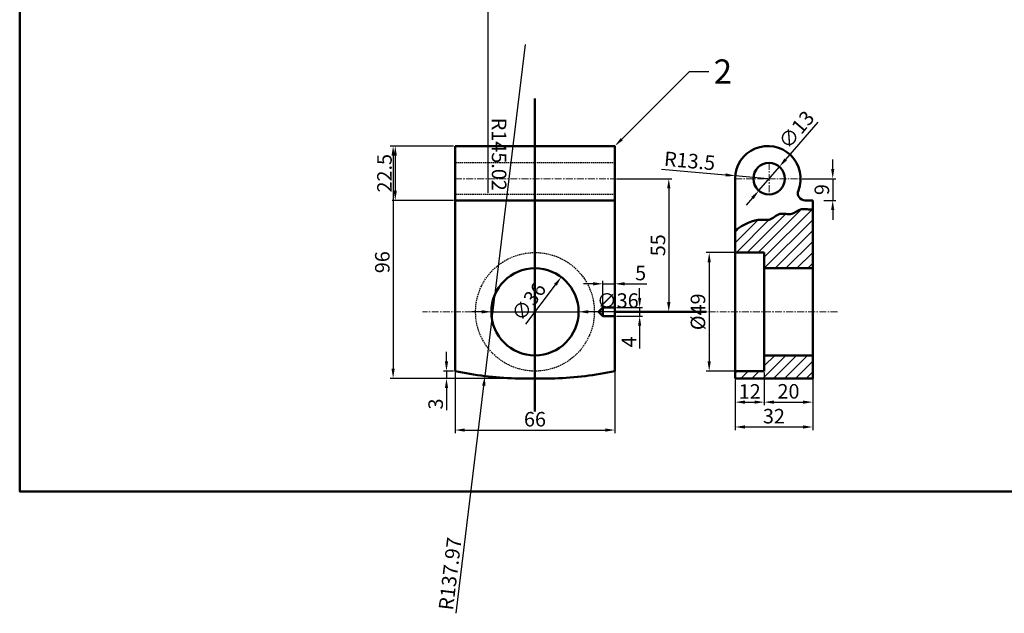
# Model space of a CAD drawing. Units: millimetres. Extents: x 197 to 841, y -182 to 351.
# Tile 1 of 3: x 197 to 603, y -182 to 63. Entities that reach past the tile are written whole.
import ezdxf
from ezdxf import colors
from ezdxf.entities.mleader import LeaderData, LeaderLine
from ezdxf.math import Vec2, Vec3

# ---------------------------------------------------------------- set-up
doc = ezdxf.new("R2010")
doc.units = ezdxf.units.MM
doc.header["$LTSCALE"] = 0.3
doc.linetypes.add('CENTER', pattern=[50.8, 31.75, -6.35, 6.35, -6.35])
doc.linetypes.add('HIDDEN', pattern=[9.525, 6.35, -3.175])
for name, color, linetype, lineweight in [('M-CNTR', 1, 'CENTER', 18), ('M-DIMS', 2, 'Continuous', 25), ('M-HATC', 8, 'Continuous', 18), ('M-HIDN', 6, 'HIDDEN', 25), ('M-OUTL', 7, 'Continuous', 50), ('M-TTLB', 7, 'Continuous', 50)]:
    doc.layers.add(name, color=color, linetype=linetype, lineweight=lineweight)
doc.styles.get("Standard").update_dxf_attribs({"font": 'arial.ttf'})
doc.dimstyles.new('ISO-25', dxfattribs={"dimtxt": 6, "dimasz": 4, "dimexe": 1.25, "dimexo": 0.625, "dimtad": 1, "dimdec": 0, "dimtxsty": 'Standard', "dimcen": 2.5, "dimadec": 0, "dimazin": 0, "dimtfac": 1, "dimtdec": 0, "dimtmove": 0, "dimatfit": 3, "dimfxl": 1, "dimarcsym": 0})

# ---------------------------------------------------------------- blocks, each defined once
blk = doc.blocks.new('*D24')
at = {"layer": 'Defpoints', "color": 0, "ltscale": 0.3, "transparency": 16777216}
for p in [(376.21, 11.02), (350.66, -84.98), (409.21, -84.98)]:
    blk.add_point(p, dxfattribs=at)
at = {"layer": 'M-DIMS', "color": 0, "lineweight": -2, "ltscale": 0.3, "transparency": 16777216}
for p, q in [((375.58, 11.02), (349.41, 11.02)), ((350.66, 7.02), (350.66, -80.98)), ((408.58, -84.98), (349.41, -84.98))]:
    blk.add_line(p, q, dxfattribs=at)
at = {"layer": 'M-DIMS', "color": 0, "ltscale": 0.3, "transparency": 16777216}
for points in [[(349.99, 7.02), (351.32, 7.02), (350.66, 11.02)], [(349.99, -80.98), (351.32, -80.98), (350.66, -84.98)]]:
    blk.add_solid(points, dxfattribs=at)
at = {"layer": 'M-DIMS', "color": 0, "ltscale": 0.3, "transparency": 16777216, "insert": (346.97, -36.98), "char_height": 6, "attachment_point": 5, "rotation": 90}
blk.add_mtext('96', dxfattribs=at)
blk = doc.blocks.new('*D25')
at = {"layer": 'Defpoints', "color": 0, "ltscale": 0.3, "transparency": 16777216}
for p in [(376.21, -72.47), (442.21, -72.47), (442.21, -106.33)]:
    blk.add_point(p, dxfattribs=at)
at = {"layer": 'M-DIMS', "color": 0, "lineweight": -2, "ltscale": 0.3, "transparency": 16777216}
for p, q in [((376.21, -73.1), (376.21, -107.58)), ((442.21, -73.1), (442.21, -107.58)), ((380.21, -106.33), (438.21, -106.33))]:
    blk.add_line(p, q, dxfattribs=at)
at = {"layer": 'M-DIMS', "color": 0, "ltscale": 0.3, "transparency": 16777216}
for points in [[(380.21, -105.66), (380.21, -107), (376.21, -106.33)], [(438.21, -105.66), (438.21, -107), (442.21, -106.33)]]:
    blk.add_solid(points, dxfattribs=at)
at = {"layer": 'M-DIMS', "color": 0, "ltscale": 0.3, "transparency": 16777216, "insert": (409.21, -102.64), "char_height": 6, "attachment_point": 5}
blk.add_mtext('66', dxfattribs=at)
blk = doc.blocks.new('*D26')
at = {"layer": 'Defpoints', "color": 0, "ltscale": 0.3, "transparency": 16777216}
for p in [(442.21, -55.73), (442.21, -59.23), (452.41, -59.23)]:
    blk.add_point(p, dxfattribs=at)
at = {"layer": 'M-DIMS', "color": 0, "lineweight": -2, "ltscale": 0.3, "transparency": 16777216}
for p, q in [((452.41, -51.73), (452.41, -47.73)), ((442.83, -55.73), (453.66, -55.73)), ((452.41, -55.73), (452.41, -59.23)), ((442.83, -59.23), (453.66, -59.23)), ((452.41, -63.23), (452.41, -72.63))]:
    blk.add_line(p, q, dxfattribs=at)
at = {"layer": 'M-DIMS', "color": 0, "ltscale": 0.3, "transparency": 16777216}
for points in [[(451.75, -51.73), (453.08, -51.73), (452.41, -55.73)], [(451.75, -63.23), (453.08, -63.23), (452.41, -59.23)]]:
    blk.add_solid(points, dxfattribs=at)
at = {"layer": 'M-DIMS', "color": 0, "ltscale": 0.3, "transparency": 16777216, "insert": (448.79, -69.93), "char_height": 6, "attachment_point": 5, "rotation": 90}
blk.add_mtext('4', dxfattribs=at)
blk = doc.blocks.new('*D27')
at = {"layer": 'Defpoints', "color": 0, "ltscale": 0.3, "transparency": 16777216}
for p in [(442.21, -45.91), (437.21, -57.48), (442.21, -57.48)]:
    blk.add_point(p, dxfattribs=at)
at = {"layer": 'M-DIMS', "color": 0, "lineweight": -2, "ltscale": 0.3, "transparency": 16777216}
for p, q in [((437.21, -56.85), (437.21, -44.66)), ((442.21, -56.85), (442.21, -44.66)), ((433.21, -45.91), (429.21, -45.91)), ((437.21, -45.91), (442.21, -45.91)), ((446.21, -45.91), (455.44, -45.91))]:
    blk.add_line(p, q, dxfattribs=at)
at = {"layer": 'M-DIMS', "color": 0, "ltscale": 0.3, "transparency": 16777216}
for points in [[(433.21, -45.24), (433.21, -46.58), (437.21, -45.91)], [(446.21, -45.24), (446.21, -46.58), (442.21, -45.91)]]:
    blk.add_solid(points, dxfattribs=at)
at = {"layer": 'M-DIMS', "color": 0, "ltscale": 0.3, "transparency": 16777216, "insert": (452.82, -42.23), "char_height": 6, "attachment_point": 5}
blk.add_mtext('5', dxfattribs=at)
blk = doc.blocks.new('*D28')
at = {"layer": 'Defpoints', "color": 0, "ltscale": 0.3, "transparency": 16777216}
for p in [(420.06, -43.12), (398.35, -71.84)]:
    blk.add_point(p, dxfattribs=at)
at = {"layer": 'M-DIMS', "color": 0, "lineweight": -2, "ltscale": 0.3, "transparency": 16777216}
blk.add_line((405.37, -62.56), (417.65, -46.31), dxfattribs=at)
at = {"layer": 'M-DIMS', "color": 0, "ltscale": 0.3, "transparency": 16777216}
blk.add_solid([(417.12, -45.91), (418.18, -46.71), (420.06, -43.12)], dxfattribs=at)
at = {"layer": 'M-DIMS', "color": 0, "ltscale": 0.3, "transparency": 16777216, "insert": (407.23, -53.71), "char_height": 6, "attachment_point": 5, "rotation": 52.908}
blk.add_mtext('∅36', dxfattribs=at)
blk = doc.blocks.new('*D29')
at = {"layer": 'Defpoints', "color": 0, "ltscale": 0.3, "transparency": 16777216}
for p in [(442.21, -2.48), (442.21, -57.48), (464.44, -57.48)]:
    blk.add_point(p, dxfattribs=at)
at = {"layer": 'M-DIMS', "color": 0, "lineweight": -2, "ltscale": 0.3, "transparency": 16777216}
for p, q in [((442.83, -2.48), (465.69, -2.48)), ((464.44, -6.48), (464.44, -53.48)), ((442.83, -57.48), (465.69, -57.48))]:
    blk.add_line(p, q, dxfattribs=at)
at = {"layer": 'M-DIMS', "color": 0, "ltscale": 0.3, "transparency": 16777216}
for points in [[(463.77, -6.48), (465.11, -6.48), (464.44, -2.48)], [(463.77, -53.48), (465.11, -53.48), (464.44, -57.48)]]:
    blk.add_solid(points, dxfattribs=at)
at = {"layer": 'M-DIMS', "color": 0, "ltscale": 0.3, "transparency": 16777216, "insert": (460.76, -29.98), "char_height": 6, "attachment_point": 5, "rotation": 90}
blk.add_mtext('55', dxfattribs=at)
blk = doc.blocks.new('*D30')
at = {"layer": 'Defpoints', "color": 0, "ltscale": 0.3, "transparency": 16777216}
for p in [(491.85, -32.98), (481.12, -81.98), (491.85, -81.98)]:
    blk.add_point(p, dxfattribs=at)
at = {"layer": 'M-DIMS', "color": 0, "lineweight": -2, "ltscale": 0.3, "transparency": 16777216}
for p, q in [((491.23, -32.98), (479.87, -32.98)), ((481.12, -36.98), (481.12, -77.98)), ((491.23, -81.98), (479.87, -81.98))]:
    blk.add_line(p, q, dxfattribs=at)
at = {"layer": 'M-DIMS', "color": 0, "ltscale": 0.3, "transparency": 16777216}
for points in [[(480.45, -36.98), (481.79, -36.98), (481.12, -32.98)], [(480.45, -77.98), (481.79, -77.98), (481.12, -81.98)]]:
    blk.add_solid(points, dxfattribs=at)
at = {"layer": 'M-DIMS', "color": 0, "ltscale": 0.3, "transparency": 16777216, "insert": (477.27, -57.48), "char_height": 6, "attachment_point": 5, "rotation": 90}
blk.add_mtext('%%C49', dxfattribs=at)
blk = doc.blocks.new('*D31')
at = {"layer": 'Defpoints', "color": 0, "ltscale": 0.3, "transparency": 16777216}
for p in [(491.85, -84.98), (503.85, -81.98), (503.85, -94.8)]:
    blk.add_point(p, dxfattribs=at)
at = {"layer": 'M-DIMS', "color": 0, "lineweight": -2, "ltscale": 0.3, "transparency": 16777216}
for p, q in [((503.85, -82.6), (503.85, -96.05)), ((491.85, -85.6), (491.85, -96.05)), ((495.85, -94.8), (499.85, -94.8))]:
    blk.add_line(p, q, dxfattribs=at)
at = {"layer": 'M-DIMS', "color": 0, "ltscale": 0.3, "transparency": 16777216}
for points in [[(495.85, -94.14), (495.85, -95.47), (491.85, -94.8)], [(499.85, -94.14), (499.85, -95.47), (503.85, -94.8)]]:
    blk.add_solid(points, dxfattribs=at)
at = {"layer": 'M-DIMS', "color": 0, "ltscale": 0.3, "transparency": 16777216, "insert": (497.85, -91.17), "char_height": 6, "attachment_point": 5}
blk.add_mtext('12', dxfattribs=at)
blk = doc.blocks.new('*D32')
at = {"layer": 'Defpoints', "color": 0, "ltscale": 0.3, "transparency": 16777216}
for p in [(491.85, -84.98), (523.85, -84.98), (523.85, -105.07)]:
    blk.add_point(p, dxfattribs=at)
at = {"layer": 'M-DIMS', "color": 0, "lineweight": -2, "ltscale": 0.3, "transparency": 16777216}
for p, q in [((491.85, -85.6), (491.85, -106.32)), ((523.85, -85.6), (523.85, -106.32)), ((495.85, -105.07), (519.85, -105.07))]:
    blk.add_line(p, q, dxfattribs=at)
at = {"layer": 'M-DIMS', "color": 0, "ltscale": 0.3, "transparency": 16777216}
for points in [[(495.85, -104.4), (495.85, -105.74), (491.85, -105.07)], [(519.85, -104.4), (519.85, -105.74), (523.85, -105.07)]]:
    blk.add_solid(points, dxfattribs=at)
at = {"layer": 'M-DIMS', "color": 0, "ltscale": 0.3, "transparency": 16777216, "insert": (507.85, -101.38), "char_height": 6, "attachment_point": 5}
blk.add_mtext('32', dxfattribs=at)
blk = doc.blocks.new('*D33')
at = {"layer": 'Defpoints', "color": 0, "ltscale": 0.3, "transparency": 16777216}
for p in [(523.85, -79.64), (503.85, -81.98), (523.85, -94.8)]:
    blk.add_point(p, dxfattribs=at)
at = {"layer": 'M-DIMS', "color": 0, "lineweight": -2, "ltscale": 0.3, "transparency": 16777216}
for p, q in [((523.85, -80.26), (523.85, -96.05)), ((503.85, -82.6), (503.85, -96.05)), ((507.85, -94.8), (519.85, -94.8))]:
    blk.add_line(p, q, dxfattribs=at)
at = {"layer": 'M-DIMS', "color": 0, "ltscale": 0.3, "transparency": 16777216}
for points in [[(507.85, -94.14), (507.85, -95.47), (503.85, -94.8)], [(519.85, -94.14), (519.85, -95.47), (523.85, -94.8)]]:
    blk.add_solid(points, dxfattribs=at)
at = {"layer": 'M-DIMS', "color": 0, "ltscale": 0.3, "transparency": 16777216, "insert": (513.85, -91.11), "char_height": 6, "attachment_point": 5}
blk.add_mtext('20', dxfattribs=at)
blk = doc.blocks.new('*D34')
at = {"layer": 'Defpoints', "color": 0, "ltscale": 0.3, "transparency": 16777216}
for p in [(518.85, -2.48), (527.85, -11.48), (532.11, -11.48)]:
    blk.add_point(p, dxfattribs=at)
at = {"layer": 'M-DIMS', "color": 0, "lineweight": -2, "ltscale": 0.3, "transparency": 16777216}
for p, q in [((532.11, 1.52), (532.11, 5.52)), ((519.48, -2.48), (533.36, -2.48)), ((532.11, -2.48), (532.11, -11.48)), ((528.48, -11.48), (533.36, -11.48)), ((532.11, -15.48), (532.11, -19.48))]:
    blk.add_line(p, q, dxfattribs=at)
at = {"layer": 'M-DIMS', "color": 0, "ltscale": 0.3, "transparency": 16777216}
for points in [[(531.45, 1.52), (532.78, 1.52), (532.11, -2.48)], [(531.45, -15.48), (532.78, -15.48), (532.11, -11.48)]]:
    blk.add_solid(points, dxfattribs=at)
at = {"layer": 'M-DIMS', "color": 0, "ltscale": 0.3, "transparency": 16777216, "insert": (528.42, -6.98), "char_height": 6, "attachment_point": 5, "rotation": 90}
blk.add_mtext('9', dxfattribs=at)
blk = doc.blocks.new('*D35')
at = {"layer": 'Defpoints', "color": 0, "ltscale": 0.3, "transparency": 16777216}
for p in [(510.09, 2.45), (501.62, -7.41)]:
    blk.add_point(p, dxfattribs=at)
at = {"layer": 'M-DIMS', "color": 0, "lineweight": -2, "ltscale": 0.3, "transparency": 16777216}
for p, q in [((525.97, 20.94), (512.69, 5.49)), ((501.62, -7.41), (510.09, 2.45)), ((499.01, -10.45), (496.41, -13.48))]:
    blk.add_line(p, q, dxfattribs=at)
at = {"layer": 'M-DIMS', "color": 0, "ltscale": 0.3, "transparency": 16777216}
for points in [[(512.19, 5.92), (513.2, 5.05), (510.09, 2.45)], [(498.51, -10.01), (499.52, -10.88), (501.62, -7.41)]]:
    blk.add_solid(points, dxfattribs=at)
at = {"layer": 'M-DIMS', "color": 0, "ltscale": 0.3, "transparency": 16777216, "insert": (517.71, 17.25), "char_height": 6, "attachment_point": 5, "rotation": 49.3529}
blk.add_mtext('∅13', dxfattribs=at)
blk = doc.blocks.new('*D36')
at = {"layer": 'Defpoints', "color": 0, "ltscale": 0.3, "transparency": 16777216}
for p in [(372.68, -84.98), (376.21, -81.98), (376.21, -84.98)]:
    blk.add_point(p, dxfattribs=at)
at = {"layer": 'M-DIMS', "color": 0, "lineweight": -2, "ltscale": 0.3, "transparency": 16777216}
for p, q in [((372.68, -77.98), (372.68, -73.98)), ((375.58, -81.98), (371.43, -81.98)), ((375.58, -84.98), (371.43, -84.98)), ((372.68, -81.98), (372.68, -84.98)), ((372.68, -88.98), (372.68, -98.16))]:
    blk.add_line(p, q, dxfattribs=at)
at = {"layer": 'M-DIMS', "color": 0, "ltscale": 0.3, "transparency": 16777216}
for points in [[(372.01, -77.98), (373.35, -77.98), (372.68, -81.98)], [(372.01, -88.98), (373.35, -88.98), (372.68, -84.98)]]:
    blk.add_solid(points, dxfattribs=at)
at = {"layer": 'M-DIMS', "color": 0, "ltscale": 0.3, "transparency": 16777216, "insert": (368.99, -95.57), "char_height": 6, "attachment_point": 5, "rotation": 90}
blk.add_mtext('3', dxfattribs=at)
blk = doc.blocks.new('*D65')
at = {"layer": 'Defpoints', "color": 0, "ltscale": 0.3, "transparency": 16777216}
for p in [(376.21, 11.02), (351.54, -11.48), (376.21, -11.48)]:
    blk.add_point(p, dxfattribs=at)
at = {"layer": 'M-DIMS', "color": 0, "lineweight": -2, "ltscale": 0.3, "transparency": 16777216}
for p, q in [((375.58, 11.02), (350.29, 11.02)), ((351.54, 7.02), (351.54, -7.48)), ((375.58, -11.48), (350.29, -11.48))]:
    blk.add_line(p, q, dxfattribs=at)
at = {"layer": 'M-DIMS', "color": 0, "ltscale": 0.3, "transparency": 16777216}
for points in [[(350.87, 7.02), (352.21, 7.02), (351.54, 11.02)], [(350.87, -7.48), (352.21, -7.48), (351.54, -11.48)]]:
    blk.add_solid(points, dxfattribs=at)
at = {"layer": 'M-DIMS', "color": 0, "ltscale": 0.3, "transparency": 16777216, "insert": (347.85, -0.23), "char_height": 6, "attachment_point": 5, "rotation": 90}
blk.add_mtext('22.5', dxfattribs=at)
blk = doc.blocks.new('*D70')
at = {"layer": 'Defpoints', "color": 0, "ltscale": 0.3, "transparency": 16777216}
for p in [(389.93, 239.64), (389.94, 94.62)]:
    blk.add_point(p, dxfattribs=at)
at = {"layer": 'M-DIMS', "color": 0, "lineweight": -2, "ltscale": 0.3, "transparency": 16777216}
for p, q in [((389.93, 239.64), (389.94, 94.62)), ((389.94, -8.31), (389.94, 90.62))]:
    blk.add_line(p, q, dxfattribs=at)
at = {"layer": 'M-DIMS', "color": 0, "ltscale": 0.3, "transparency": 16777216}
blk.add_solid([(390.6, 90.62), (389.27, 90.62), (389.94, 94.62)], dxfattribs=at)
at = {"layer": 'M-DIMS', "color": 0, "ltscale": 0.3, "transparency": 16777216, "insert": (393.62, 7.61), "char_height": 6, "attachment_point": 5, "rotation": 270.0001}
blk.add_mtext('R145.02', dxfattribs=at)
blk = doc.blocks.new('*D75')
at = {"layer": 'Defpoints', "color": 0, "ltscale": 0.3, "transparency": 16777216}
for p in [(391.21, -57.48), (427.21, -57.48)]:
    blk.add_point(p, dxfattribs=at)
at = {"layer": 'M-DIMS', "color": 0, "lineweight": -2, "ltscale": 0.3, "transparency": 16777216}
for p, q in [((387.21, -57.48), (383.21, -57.48)), ((391.21, -57.48), (427.21, -57.48)), ((451.58, -57.48), (431.21, -57.48))]:
    blk.add_line(p, q, dxfattribs=at)
at = {"layer": 'M-DIMS', "color": 0, "ltscale": 0.3, "transparency": 16777216}
for points in [[(387.21, -56.81), (387.21, -58.15), (391.21, -57.48)], [(431.21, -56.81), (431.21, -58.15), (427.21, -57.48)]]:
    blk.add_solid(points, dxfattribs=at)
at = {"layer": 'M-DIMS', "color": 0, "ltscale": 0.3, "transparency": 16777216, "insert": (443.39, -53.62), "char_height": 6, "attachment_point": 5, "rotation": 0.0012}
blk.add_mtext('∅36', dxfattribs=at)
blk = doc.blocks.new('*D76')
at = {"layer": 'Defpoints', "color": 0, "ltscale": 0.3, "transparency": 16777216}
for p in [(405.11, 52.93), (388.54, -84.04)]:
    blk.add_point(p, dxfattribs=at)
at = {"layer": 'M-DIMS', "color": 0, "lineweight": -2, "ltscale": 0.3, "transparency": 16777216}
for p, q in [((405.11, 52.93), (388.54, -84.04)), ((376.68, -182.06), (388.06, -88.01))]:
    blk.add_line(p, q, dxfattribs=at)
at = {"layer": 'M-DIMS', "color": 0, "ltscale": 0.3, "transparency": 16777216}
blk.add_solid([(387.4, -87.93), (388.72, -88.09), (388.54, -84.04)], dxfattribs=at)
at = {"layer": 'M-DIMS', "color": 0, "ltscale": 0.3, "transparency": 16777216, "insert": (374.94, -165.78), "char_height": 6, "attachment_point": 5, "rotation": 83.1031}
blk.add_mtext('R137.97', dxfattribs=at)
blk = doc.blocks.new('*D77')
at = {"layer": 'Defpoints', "color": 0, "ltscale": 0.3, "transparency": 16777216}
for p in [(491.91, -1.28), (505.35, -2.48)]:
    blk.add_point(p, dxfattribs=at)
at = {"layer": 'M-DIMS', "color": 0, "lineweight": -2, "ltscale": 0.3, "transparency": 16777216}
for p, q in [((461.41, 1.45), (487.92, -0.92)), ((505.35, -2.48), (491.91, -1.28))]:
    blk.add_line(p, q, dxfattribs=at)
at = {"layer": 'M-DIMS', "color": 0, "ltscale": 0.3, "transparency": 16777216}
blk.add_solid([(487.98, -0.26), (487.86, -1.59), (491.91, -1.28)], dxfattribs=at)
at = {"layer": 'M-DIMS', "color": 0, "ltscale": 0.3, "transparency": 16777216, "insert": (473, 4.12), "char_height": 6, "attachment_point": 5, "rotation": 354.8911}
blk.add_mtext('R13.5', dxfattribs=at)

msp = doc.modelspace()

# ---------------------------------------------------------------- hatches: boundary and pattern name
at = {"layer": 'M-HATC', "ltscale": 0.3}
h = msp.add_hatch(dxfattribs=at)
h.set_pattern_fill('ANSI31', color=256)
edge = h.paths.add_edge_path()
edge.add_spline(control_points=[(523.8547, -15.1343), (523.0917, -15.1567), (521.5464, -15.2021), (518.4208, -14.7543), (515.2877, -18.1529), (509.9543, -15.8649), (506.669, -19.9832), (499.7493, -18.6745), (495.3559, -21.5359), (491.8547, -23.8162)], knot_values=[0, 0, 0, 0, 2.30450902, 4.66737561, 9.06571731, 14.06619701, 19.00763742, 22.02990433, 33.88867978, 33.88867978, 33.88867978, 33.88867978], degree=3, periodic=0)
edge.add_line((491.8547, -23.8162), (491.8547, -32.9794))
edge.add_line((491.8547, -32.9794), (503.8547, -32.9794))
edge.add_line((503.8547, -32.9794), (503.8547, -39.4794))
edge.add_line((503.8547, -39.4794), (523.8547, -39.4794))
edge.add_line((523.8547, -39.4794), (523.8547, -15.1343))
h.paths.add_polyline_path([(523.8547, -75.4794), (503.8547, -75.4794), (503.8547, -81.9794), (491.8547, -81.9794), (491.8547, -84.9794), (507.8547, -84.9794), (523.8547, -84.9794)])

# ---------------------------------------------------------------- linework, layer by layer
at = {"layer": 'M-CNTR', "ltscale": 0.3}
for p, q in [((505.8547, 4.0206), (505.8547, -8.9794)), ((376.2072, -2.4794), (442.2072, -2.4794)), ((491.8547, -2.4794), (518.8547, -2.4794)), ((534.0295, -57.4794), (362.791, -57.4794))]:
    msp.add_line(p, q, dxfattribs=at)
at = {"layer": 'M-HIDN', "ltscale": 0.3}
for p, q in [((442.2072, 4.0206), (376.2072, 4.0206)), ((442.2072, -8.9794), (376.2072, -8.9794))]:
    msp.add_line(p, q, dxfattribs=at)
msp.add_circle((409.2072, -57.4794), 24.5, dxfattribs=at)
at = {"layer": 'M-OUTL', "ltscale": 0.3}
for p, q in [((409.2072, 30.6574), (409.2072, -98.6488)), ((376.2072, 11.0206), (376.2072, -81.9794)), ((442.2072, 11.0206), (376.2072, 11.0206)), ((442.2072, -81.9794), (442.2072, 11.0206)), ((505.3547, 11.0206), (505.8547, 11.0206)), ((505.8547, 11.0206), (505.8547, 11.0113)), ((491.8547, -84.9794), (491.8547, -2.4794)), ((376.2072, -11.4794), (442.2072, -11.4794)), ((520.7251, -11.4794), (523.8547, -11.4794)), ((523.8547, -84.9794), (523.8547, -11.4794)), ((491.8547, -32.9794), (503.8547, -32.9794)), ((503.8547, -81.9794), (503.8547, -32.9794)), ((503.8547, -39.4794), (523.8547, -39.4794)), ((437.2072, -55.7294), (435.4572, -57.4794)), ((437.2072, -55.7294), (442.2072, -55.7294)), ((437.2072, -59.2294), (437.2072, -55.7294)), ((442.2072, -55.7294), (442.2072, -59.2294)), ((437.2072, -59.2294), (435.4572, -57.4794)), ((442.2072, -59.2294), (437.2072, -59.2294)), ((442.2072, -57.4794), (479.8547, -57.4794)), ((503.8547, -75.4794), (523.8547, -75.4794)), ((401.0097, -84.9794), (417.4048, -84.9794)), ((491.8547, -81.9794), (503.8547, -81.9794)), ((507.8547, -84.9794), (491.8547, -84.9794)), ((507.8547, -84.9794), (523.8547, -84.9794))]:
    msp.add_line(p, q, dxfattribs=at)
for centre, radius in [((505.8547, -2.4794), 6.5), ((409.2072, -57.4794), 18)]:
    msp.add_circle(centre, radius, dxfattribs=at)
for centre, radius, start, end in [((505.3547, -2.4794), 13.5, 338.676314, 180), ((520.7251, -8.4794), 3, 158.676314, 270), ((405.1085, 52.934), 137.9743, 257.908816, 268.297674), ((413.306, 52.934), 137.9743, 271.702326, 282.091184)]:
    msp.add_arc(centre, radius, start, end, dxfattribs=at)
msp.add_open_spline([(491.8547, -23.8162), (495.3559, -21.5359), (499.7493, -18.6745), (506.669, -19.9832), (509.9543, -15.8649), (515.2877, -18.1529), (518.4208, -14.7543), (521.5464, -15.2021), (523.0917, -15.1567), (523.8547, -15.1343)], degree=3, knots=[0, 0, 0, 0, 11.85877546, 14.88104237, 19.82248277, 24.82296247, 29.22130417, 31.58417077, 33.88867978, 33.88867978, 33.88867978, 33.88867978], dxfattribs=at)
at = {"layer": 'M-TTLB', "ltscale": 0.3}
msp.add_lwpolyline([(196.5121, 350.7597), (840.9228, 350.7597), (840.9228, -131.7005), (196.5121, -131.7005)], close=True, dxfattribs=at)

# ---------------------------------------------------------------- dimensions: what is measured, and where the dimension line sits
at = {"layer": 'M-DIMS', "ltscale": 0.3}
for center, mpoint, picture, middle in [((389.9348, 239.6364), (389.935, 94.6207), '*D70', (389.9351, 7.6114)), ((405.1085, 52.934), (388.54, -84.0419), '*D76', (378.5989, -166.2274))]:
    dim = msp.add_radius_dim(center=center, mpoint=mpoint, dimstyle='ISO-25', override={"dimdec": 2, "dimlfac": 1, "dimrnd": 0, "dimzin": 0, "dimdsep": 46, "dimlunit": 2}, dxfattribs=at)
    dim.commit()
    dim.dimension.update_dxf_attribs({"geometry": picture, "text_midpoint": middle, "dimtype": 164})
for p1, p2, override, picture, middle in [((501.6206, -7.4112), (510.0887, 2.4524), {"dimclrd": 0, "dimclre": 0, "dimclrt": 0}, '*D35', (517.7067, 17.2455)), ((391.2072, -57.4798), (427.2072, -57.479), {"dimdec": 0, "dimlfac": 1, "dimrnd": 0, "dimzin": 0, "dimdsep": 46, "dimlunit": 2}, '*D75', (443.3916, -57.4786))]:
    dim = msp.add_diameter_dim_2p(p1=p1, p2=p2, dimstyle='ISO-25', override=override, dxfattribs=at)
    dim.commit()
    dim.dimension.update_dxf_attribs({"geometry": picture, "text_midpoint": middle})
for base, p1, p2, override, picture, middle in [((350.6559, -84.9794), (376.2072, 11.0206), (409.2072, -84.9794), {"dimclrd": 0, "dimclre": 0, "dimclrt": 0}, '*D24', (346.9675, -36.9794)), ((351.541, -11.4794), (376.2072, 11.0206), (376.2072, -11.4794), {"dimdec": 1, "dimlfac": 1, "dimrnd": 0, "dimzin": 0, "dimdsep": 46, "dimlunit": 2}, '*D65', (347.8526, -0.2294)), ((532.1122, -11.4794), (518.8547, -2.4794), (527.8547, -11.4794), {"dimclrd": 0, "dimclre": 0, "dimclrt": 0}, '*D34', (528.4238, -6.9794)), ((464.441, -57.4794), (442.2072, -2.4794), (442.2072, -57.4794), {"dimclrd": 0, "dimclre": 0, "dimclrt": 0}, '*D29', (460.7648, -29.9794)), ((452.4137115755, -59.2293913813), (442.2072408596, -55.7293913813), (442.2072408596, -59.2293913813), {"dimclrd": 0, "dimclre": 0, "dimclrt": 0}, '*D26', (448.7887115755, -69.9294254877)), ((372.6785, -84.9794), (376.2072, -81.9794), (376.2072, -84.9794), {"dimclrd": 0, "dimclre": 0, "dimclrt": 0}, '*D36', (368.988, -95.5689))]:
    dim = msp.add_linear_dim(base=base, p1=p1, p2=p2, angle=90, dimstyle='ISO-25', override=override, dxfattribs=at)
    dim.commit()
    dim.dimension.update_dxf_attribs({"geometry": picture, "text_midpoint": middle})
dim = msp.add_radius_dim(center=(505.3547, -2.4794), mpoint=(491.9083, -1.2772), dimstyle='ISO-25', override={"dimdec": 1, "dimlfac": 1, "dimrnd": 0, "dimzin": 0, "dimdsep": 46, "dimlunit": 2}, dxfattribs=at)
dim.commit()
dim.dimension.update_dxf_attribs({"geometry": '*D77', "text_midpoint": (473.0024, 4.1182)})
dim = msp.add_linear_dim(base=(481.1213, -81.9794), p1=(491.8547, -32.9794), p2=(491.8547, -81.9794), angle=90, text='%%C<>', dimstyle='ISO-25', override={"dimclrd": 0, "dimclre": 0, "dimclrt": 0}, dxfattribs=at)
dim.commit()
dim.dimension.update_dxf_attribs({"geometry": '*D30', "text_midpoint": (477.265, -57.4794)})
for base, p1, p2, picture, middle in [((442.2072, -45.9084), (437.2072, -57.4794), (442.2072, -57.4794), '*D27', (452.8213, -42.2323)), ((442.2072, -106.3293), (376.2072, -72.4722), (442.2072, -72.4722), '*D25', (409.2072, -102.6409)), ((523.8547, -94.8031), (503.8547, -81.9794), (523.8547, -79.6399), '*D33', (513.8547, -91.1147)), ((503.8547, -94.8031), (491.8547, -84.9794), (503.8547, -81.9794), '*D31', (497.8547, -91.1658)), ((523.8547, -105.0688), (491.8547, -84.9794), (523.8547, -84.9794), '*D32', (507.8547, -101.3783))]:
    dim = msp.add_linear_dim(base=base, p1=p1, p2=p2, dimstyle='ISO-25', override={"dimclrd": 0, "dimclre": 0, "dimclrt": 0}, dxfattribs=at)
    dim.commit()
    dim.dimension.update_dxf_attribs({"geometry": picture, "text_midpoint": middle})
dim = msp.add_diameter_dim_2p(p1=(398.3515, -71.8374), p2=(420.063, -43.1214), dimstyle='ISO-25', override={"dimclrd": 0, "dimclre": 0, "dimclrt": 0}, dxfattribs=at)
dim.commit()
dim.dimension.update_dxf_attribs({"geometry": '*D28', "text_midpoint": (410.3023, -56.0311), "dimtype": 163})

# ---------------------------------------------------------------- leaders
ml = msp.add_multileader_mtext('Standard', dxfattribs=at)
ml.set_content('2', color=256)
ml.set_leader_properties()
ml.build(insert=Vec2(0, 0))
ctx = ml.context
ctx.base_point, ctx.char_height, ctx.plane_origin = Vec3(480.9914, 41.8048), 10, Vec3(442.2072, 11.0206)
notes = []
notes.append((ctx, [(0, (1, 1, 0), (472.9914, 41.8048), (1, 0), 8, [(0, [(442.2072, 11.0206)], 0, [])])]))
ctx.mtext.insert, ctx.mtext.flow_direction = Vec3(482.9914, 46.8048), 5
for ctx, leaders in notes:
    for number, flags, end, landing, length, lines in leaders:
        leader = LeaderData()
        leader.index, (leader.has_last_leader_line, leader.has_dogleg_vector, leader.attachment_direction) = number, flags
        leader.last_leader_point, leader.dogleg_vector, leader.dogleg_length = Vec3(end), Vec3(landing), length
        for number, points, colour, breaks in lines:
            line = LeaderLine()
            line.index, line.vertices, line.color, line.breaks = number, Vec3.list(points), colors.encode_raw_color(colour), breaks
            leader.lines.append(line)
        ctx.leaders.append(leader)

doc.saveas('drawing.dxf')
